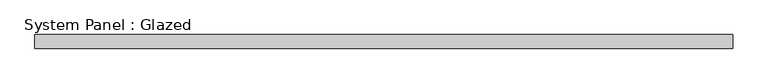
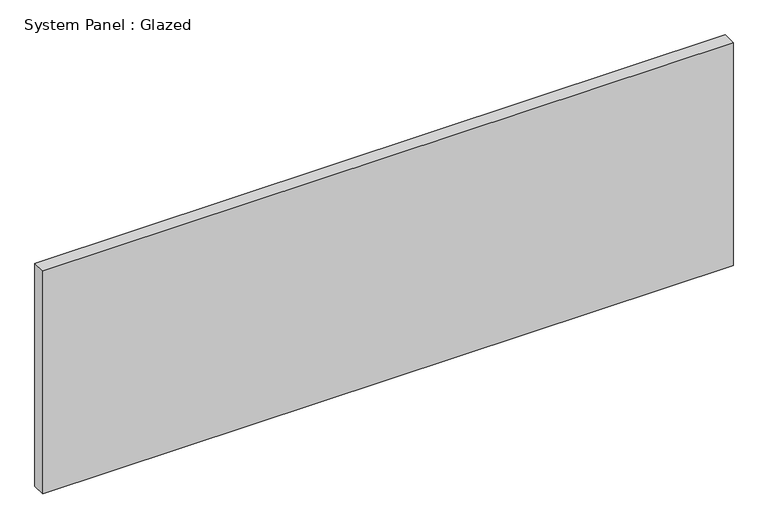
"""IFC4 building model written with IfcOpenShell, lengths in millimetres: plate geometry, System Panel : Glazed."""

from ifc_helpers import new_model, si_unit, origin, origin_with_axes, place, context, project, spatial, polyline, outline, extrude, source, transform, mapped, element, save


def system_panel_glazed_b8338f5c(model_context):
    return source(origin(), model_context, "Body", "SweptSolid", [
        extrude(outline(polyline([(650.8750001, -44.45), (-650.8750001, -44.45), (-650.8750001, -19.05), (650.8750001, -19.05), (650.8750001, -44.45)])), origin_with_axes(), (0.0, 0.0, 1.0), 444.5),
    ])


if __name__ == "__main__":
    model = new_model("IFC4")
    model_context = context("Model", 3, world=origin())
    ifc_project = project(units=[si_unit("LENGTHUNIT", "METRE", prefix="MILLI")], contexts=[model_context])
    site = spatial("IfcSite", under=ifc_project)
    building = spatial("IfcBuilding", under=site)
    placement = place(None, origin())
    system_panel_glazed_shape = system_panel_glazed_b8338f5c(model_context)
    element("IfcPlate", 1, ObjectType="System Panel : Glazed", at=placement, inside=building, context=model_context, shape_type="MappedRepresentation", body=[
        mapped(system_panel_glazed_shape, transform((0.0, 0.0, 0.0), x_axis=(1.0, 0.0, 0.0), y_axis=(0.0, 1.0, 0.0), z_axis=(0.0, 0.0, 1.0))),
    ])
    save(model, "model.ifc")

# Revit data of these elements
# Type "System Panel : Glazed"
#   Construction Type Id = "GSP4R"
#   Analytic Construction = "1/8 in Pilkington single glazing"
#   Visual Light Transmittance = 0.9
#   Solar Heat Gain Coefficient = 0.86
#   Heat Transfer Coefficient (U) = 1.18115 BTU/(h·ft²·°F)
#   Define Thermal Properties by = 1
# Element 1 (IfcPlate, "System Panel : Glazed")
#   Materials on its faces: "glass panel 223"
# Materials
#   "glass panel 223": class "Generic", colour RGB 120 120 120, transparency 0, Cost = 0
